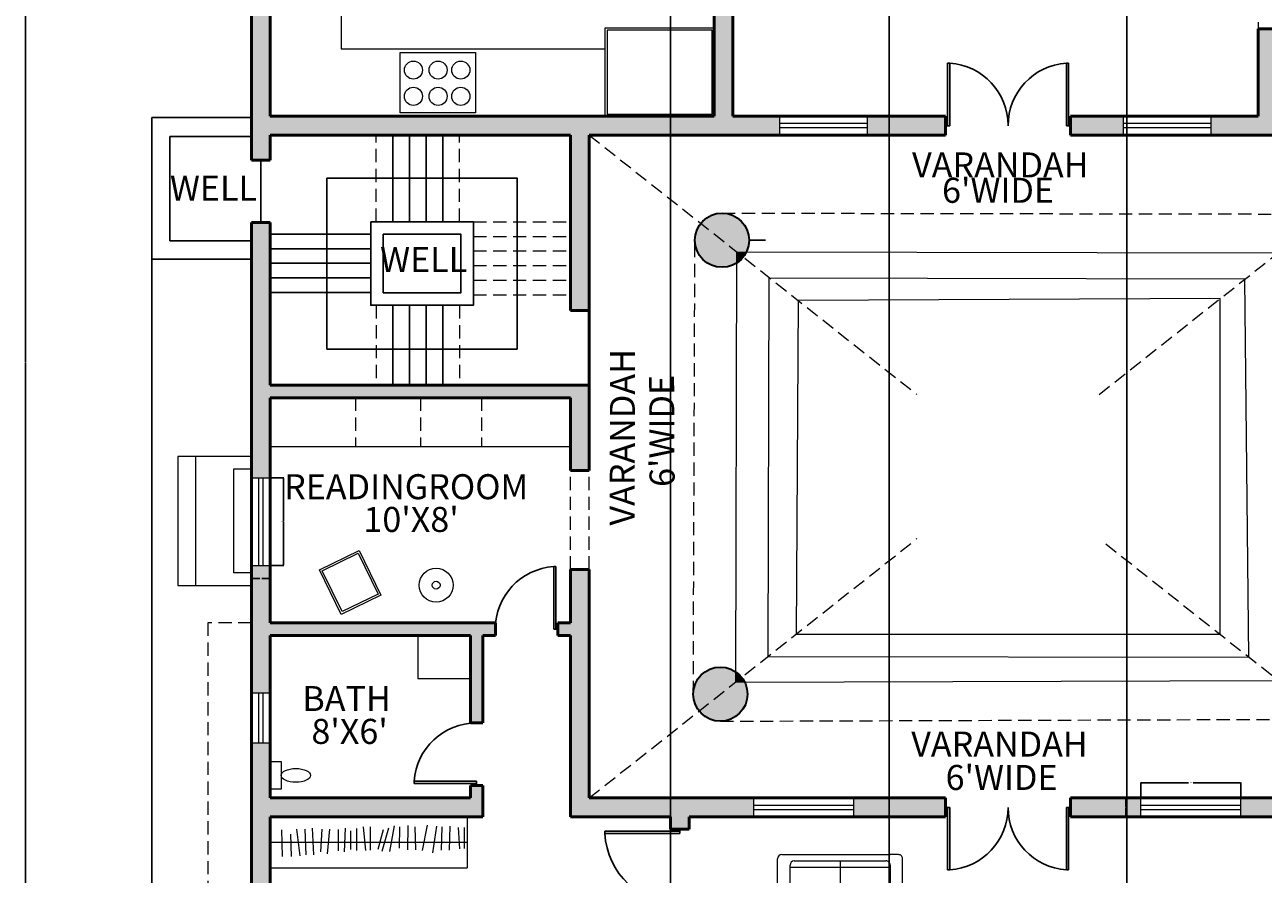
# Model space of a CAD drawing. Units: inches. Extents: x 2743 to 3669, y 1014 to 2282.
# Tile 2 of 5: x 2743 to 3337, y 1403 to 1810. Entities that reach past the tile are written whole.
import ezdxf

# ---------------------------------------------------------------- set-up
doc = ezdxf.new("R2010")
doc.units = ezdxf.units.IN
doc.linetypes.add('DASHED2', pattern=[9.525, 6.35, -3.175])
for name, color, linetype, lineweight in [('A-ANNO-DIMS', 2, 'Continuous', 18), ('A-ANNO-TEXT', 4, 'Continuous', 18), ('A-AREA-IDEN', 4, 'Continuous', 18), ('A-COLS', 7, 'Continuous', 35), ('A-DOOR', 211, 'Continuous', 25), ('A-EQPM', 51, 'Continuous', 18), ('A-FLOR-CASE', 51, 'Continuous', 18), ('A-FLOR-CASE-OVHD', 8, 'DASHED2', 13), ('A-FLOR-STRS', 7, 'Continuous', 25), ('A-FLOR-STRS-OVHD', 8, 'DASHED2', 18), ('A-FURN', 111, 'Continuous', 18), ('A-GLAZ', 40, 'Continuous', 20), ('A-ROOF', 7, 'Continuous', 20), ('A-ROOF-OVHD', 8, 'DASHED2', 18), ('A-WALL', 7, 'Continuous', 50), ('A-WALL-OVHD', 8, 'DASHED2', 18), ('P-EQPM', 4, 'Continuous', 25)]:
    doc.layers.add(name, color=color, linetype=linetype, lineweight=lineweight)
for name, color, linetype, lineweight, true_color in [('A-COLS-PATT', 47, 'Continuous', 13, 0x726c55), ('A-FLOR-FIXT', 11, 'Continuous', 18, 0xee778f), ('A-WALL-PATT', 47, 'Continuous', 13, 0x726c55)]:
    doc.layers.add(name, color=color, linetype=linetype, lineweight=lineweight, true_color=true_color)
doc.styles.get("Standard").update_dxf_attribs({"font": 'arial.ttf'})
doc.dimstyles.get("Standard").update_dxf_attribs({"dimtxt": 0.18, "dimasz": 0.18, "dimexe": 0.18, "dimexo": 0.0625, "dimgap": 0.09, "dimtad": 0, "dimtih": 1, "dimtoh": 1, "dimdec": 4, "dimzin": 0, "dimdsep": 46, "dimtxsty": 'Standard', "dimcen": 0.09, "dimadec": 0, "dimazin": 0, "dimtfac": 1, "dimtdec": 4, "dimtofl": 0, "dimtmove": 0, "dimatfit": 3, "dimfxl": 1, "dimtolj": 1, "dimtzin": 0, "dimarcsym": 0})

# ---------------------------------------------------------------- blocks, each defined once
blk = doc.blocks.new('DOOR-PAIR-60IN')
for p, q in [((0, 30), (1, 30)), ((1, 30), (1, 0)), ((2, 30), (1, 30)), ((2, 0), (2, 30)), ((58, 0), (58, 30)), ((58, 30), (59, 30)), ((60, 30), (59, 30)), ((59, 30), (59, 0)), ((1, 0), (2, 0)), ((59, 0), (58, 0))]:
    blk.add_line(p, q)
for centre, start, end in [((0, 29.93), 273.82241, 0.12746), ((60, 29.93), 179.99998, 266.1773)]:
    blk.add_arc(centre, 30, start, end)
blk = doc.blocks.new('DOOR-SINGLE-30IN')
for p, q in [((1, 0), (1, 30)), ((1, 30), (2, 30)), ((2, 30), (2, 0)), ((0, 0), (1, 0)), ((2, 0), (1, 0))]:
    blk.add_line(p, q)
blk.add_arc((0, 0.07), 30, 359.87254, 86.17759)
blk = doc.blocks.new('DOOR-SINGLE-36IN')
for p, q in [((1, 0), (1, 36)), ((1, 36), (2, 36)), ((2, 36), (2, 0)), ((0, 0), (1, 0)), ((2, 0), (1, 0))]:
    blk.add_line(p, q)
blk.add_arc((0, 0.06), 36, 359.91152, 86.81533)
blk = doc.blocks.new('WINDOW-24IN')
for p, q in [((0, 9), (0, 0)), ((24, 9), (24, 0)), ((0, 5.5), (24, 5.5)), ((0, 3.5), (24, 3.5))]:
    blk.add_line(p, q)
blk = doc.blocks.new('WINDOW-42IN')
for p, q in [((0, 42), (9, 42)), ((3.5, 0), (3.5, 42)), ((5.5, 0), (5.5, 42)), ((0, 0), (9, 0))]:
    blk.add_line(p, q)
blk = doc.blocks.new('WINDOW-48IN')
for p, q in [((0, 0), (0, 9)), ((48, 0), (48, 9)), ((0, 5.5), (48, 5.5)), ((0, 3.5), (48, 3.5))]:
    blk.add_line(p, q)
blk = doc.blocks.new('SOFA-TWO-SEAT')
for p, q in [((5, 60), (31, 60)), ((2, 54), (28, 54)), ((3, 54), (3, 58)), ((27, 54), (27, 6)), ((33, 58), (33, 6)), ((0, 32), (0, 52)), ((30, 52), (30, 8)), ((30, 30), (2, 30)), ((2, 30), (2, 30)), ((0, 28), (0, 8)), ((28, 6), (2, 6)), ((2, 6), (2, 6)), ((3, 6), (3, 2)), ((33, 2), (33, 6)), ((5, 0), (31, 0))]:
    blk.add_line(p, q)
for centre, start, end in [((5, 58), 90, 180), ((31, 58), 0, 90), ((2, 52), 90, 180), ((28, 52), 0, 90), ((2, 32), 180, 270), ((2, 28), 90, 180), ((2, 8), 180, 270), ((28, 8), 270, 0), ((5, 2), 180, 270), ((31, 2), 270, 0)]:
    blk.add_arc(centre, 2, start, end)
blk = doc.blocks.new('WC')
blk.add_lwpolyline([(0, 13.38), (5.3, 13.38), (5.3, 0), (0, 0)], close=True)
blk.add_ellipse((12.29, 6.69), major_axis=(7.08, 0), ratio=0.464281)
blk = doc.blocks.new('POST-COURTYARD')
blk.add_circle((13, 13), 13)
blk = doc.blocks.new('*D36')
at = {"layer": 'A-ANNO-DIMS', "color": 0, "lineweight": -2, "transparency": 16777216}
for p, q in [((2860.86, 1592.68), (2867.28, 1592.68)), ((2867.1, 1592.5), (2867.1, 1571.86)), ((2867.1, 1550.86), (2867.1, 1571.5)), ((2860.86, 1550.68), (2867.28, 1550.68))]:
    blk.add_line(p, q, dxfattribs=at)
at = {"layer": 'A-ANNO-DIMS', "color": 0, "transparency": 16777216}
for points in [[(2867.07, 1592.5), (2867.13, 1592.5), (2867.1, 1592.68)], [(2867.07, 1550.86), (2867.13, 1550.86), (2867.1, 1550.68)]]:
    blk.add_solid(points, dxfattribs=at)
at = {"layer": 'Defpoints', "color": 0, "transparency": 16777216}
for p in [(2860.8, 1592.68), (2867.1, 1592.68), (2860.8, 1550.68)]:
    blk.add_point(p, dxfattribs=at)
at = {"layer": 'A-ANNO-DIMS', "color": 0, "transparency": 16777216, "insert": (2867.1, 1571.68), "char_height": 0.18, "attachment_point": 5}
blk.add_mtext('\\A1;WINDOW 42 TYP.', dxfattribs=at)
blk = doc.blocks.new('*D37')
at = {"layer": 'A-ANNO-DIMS', "color": 0, "lineweight": -2, "transparency": 16777216}
for p, q in [((2851.8, 1550.62), (2851.8, 1544.2)), ((2860.8, 1550.62), (2860.8, 1544.2)), ((2851.98, 1544.38), (2855.84, 1544.38)), ((2860.62, 1544.38), (2856.75, 1544.38))]:
    blk.add_line(p, q, dxfattribs=at)
at = {"layer": 'A-ANNO-DIMS', "color": 0, "transparency": 16777216}
for points in [[(2851.98, 1544.41), (2851.98, 1544.35), (2851.8, 1544.38)], [(2860.62, 1544.41), (2860.62, 1544.35), (2860.8, 1544.38)]]:
    blk.add_solid(points, dxfattribs=at)
at = {"layer": 'Defpoints', "color": 0, "transparency": 16777216}
for p in [(2851.8, 1550.68), (2860.8, 1550.68), (2860.8, 1544.38)]:
    blk.add_point(p, dxfattribs=at)
at = {"layer": 'A-ANNO-DIMS', "color": 0, "transparency": 16777216, "insert": (2856.3, 1544.38), "char_height": 0.18, "attachment_point": 5}
blk.add_mtext('\\A1;9 TYP.', dxfattribs=at)
blk = doc.blocks.new('*D50')
at = {"layer": 'A-ANNO-DIMS', "color": 0, "lineweight": -2, "transparency": 16777216}
for p, q in [((3278.44, 1439.16), (3278.44, 1446.47)), ((3278.62, 1446.29), (3301.32, 1446.29)), ((3326.26, 1446.29), (3303.56, 1446.29)), ((3326.44, 1439.16), (3326.44, 1446.47))]:
    blk.add_line(p, q, dxfattribs=at)
at = {"layer": 'A-ANNO-DIMS', "color": 0, "transparency": 16777216}
for points in [[(3278.62, 1446.32), (3278.62, 1446.26), (3278.44, 1446.29)], [(3326.26, 1446.32), (3326.26, 1446.26), (3326.44, 1446.29)]]:
    blk.add_solid(points, dxfattribs=at)
at = {"layer": 'Defpoints', "color": 0, "transparency": 16777216}
for p in [(3326.44, 1446.29), (3278.44, 1439.09), (3326.44, 1439.09)]:
    blk.add_point(p, dxfattribs=at)
at = {"layer": 'A-ANNO-DIMS', "color": 0, "transparency": 16777216, "insert": (3302.44, 1446.29), "char_height": 0.18, "attachment_point": 5}
blk.add_mtext('\\A1;WINDOW 48 TYP.', dxfattribs=at)
blk = doc.blocks.new('*D51')
at = {"layer": 'A-ANNO-DIMS', "color": 0, "lineweight": -2, "transparency": 16777216}
for p, q in [((3278.38, 1439.09), (3271.06, 1439.09)), ((3271.24, 1438.91), (3271.24, 1434.78)), ((3271.24, 1430.27), (3271.24, 1434.41)), ((3278.38, 1430.09), (3271.06, 1430.09))]:
    blk.add_line(p, q, dxfattribs=at)
at = {"layer": 'A-ANNO-DIMS', "color": 0, "transparency": 16777216}
for points in [[(3271.21, 1438.91), (3271.27, 1438.91), (3271.24, 1439.09)], [(3271.21, 1430.27), (3271.27, 1430.27), (3271.24, 1430.09)]]:
    blk.add_solid(points, dxfattribs=at)
at = {"layer": 'Defpoints', "color": 0, "transparency": 16777216}
for p in [(3271.24, 1439.09), (3278.44, 1439.09), (3278.44, 1430.09)]:
    blk.add_point(p, dxfattribs=at)
at = {"layer": 'A-ANNO-DIMS', "color": 0, "transparency": 16777216, "insert": (3271.24, 1434.59), "char_height": 0.18, "attachment_point": 5}
blk.add_mtext('\\A1;9 TYP.', dxfattribs=at)
blk = doc.blocks.new('*D62')
at = {"layer": 'A-ANNO-DIMS', "color": 0, "lineweight": -2, "transparency": 16777216}
for p, q in [((3608.38, 1899.55), (3608.38, 1014.41)), ((2803.91, 1765.52), (2803.91, 1014.41)), ((2804.09, 1014.59), (3205.75, 1014.59)), ((3608.2, 1014.59), (3206.54, 1014.59))]:
    blk.add_line(p, q, dxfattribs=at)
at = {"layer": 'A-ANNO-DIMS', "color": 0, "transparency": 16777216}
for points in [[(2804.09, 1014.62), (2804.09, 1014.56), (2803.91, 1014.59)], [(3608.2, 1014.62), (3608.2, 1014.56), (3608.38, 1014.59)]]:
    blk.add_solid(points, dxfattribs=at)
at = {"layer": 'Defpoints', "color": 0, "transparency": 16777216}
for p in [(3608.38, 1899.61), (2803.91, 1765.58), (3608.38, 1014.59)]:
    blk.add_point(p, dxfattribs=at)
at = {"layer": 'A-ANNO-DIMS', "color": 0, "transparency": 16777216, "insert": (3206.15, 1014.59), "char_height": 0.18, "attachment_point": 5}
blk.add_mtext('\\A1;804.5', dxfattribs=at)
blk = doc.blocks.new('*D63')
at = {"layer": 'A-ANNO-DIMS', "color": 0, "lineweight": -2, "transparency": 16777216}
for p, q in [((3001.57, 2220.87), (2743.18, 2220.87)), ((2743.36, 2220.69), (2743.36, 1648.19)), ((2743.36, 1075.32), (2743.36, 1647.82)), ((3214.73, 1075.14), (2743.18, 1075.14))]:
    blk.add_line(p, q, dxfattribs=at)
at = {"layer": 'A-ANNO-DIMS', "color": 0, "transparency": 16777216}
for points in [[(2743.33, 2220.69), (2743.39, 2220.69), (2743.36, 2220.87)], [(2743.33, 1075.32), (2743.39, 1075.32), (2743.36, 1075.14)]]:
    blk.add_solid(points, dxfattribs=at)
at = {"layer": 'Defpoints', "color": 0, "transparency": 16777216}
for p in [(2743.36, 2220.87), (3001.63, 2220.87), (3214.8, 1075.14)]:
    blk.add_point(p, dxfattribs=at)
at = {"layer": 'A-ANNO-DIMS', "color": 0, "transparency": 16777216, "insert": (2743.36, 1648.01), "char_height": 0.18, "attachment_point": 5}
blk.add_mtext('\\A1;1145.7', dxfattribs=at)
blk = doc.blocks.new('*D76')
at = {"layer": 'A-ANNO-DIMS', "color": 0, "lineweight": -2, "transparency": 16777216}
for p, q in [((3052.84, 1130.9), (3052.84, 2281.6)), ((3053.02, 2281.42), (3104.86, 2281.42)), ((3157.62, 2281.42), (3105.77, 2281.42)), ((3157.8, 1130.9), (3157.8, 2281.6))]:
    blk.add_line(p, q, dxfattribs=at)
at = {"layer": 'A-ANNO-DIMS', "color": 0, "transparency": 16777216}
for points in [[(3053.02, 2281.45), (3053.02, 2281.39), (3052.84, 2281.42)], [(3157.62, 2281.45), (3157.62, 2281.39), (3157.8, 2281.42)]]:
    blk.add_solid(points, dxfattribs=at)
at = {"layer": 'Defpoints', "color": 0, "transparency": 16777216}
for p in [(3157.8, 2281.42), (3052.84, 1130.83), (3157.8, 1130.83)]:
    blk.add_point(p, dxfattribs=at)
at = {"layer": 'A-ANNO-DIMS', "color": 0, "transparency": 16777216, "insert": (3105.32, 2281.42), "char_height": 0.18, "attachment_point": 5}
blk.add_mtext('\\A1;104.95', dxfattribs=at)
blk = doc.blocks.new('*D77')
at = {"layer": 'A-ANNO-DIMS', "color": 0, "lineweight": -2, "transparency": 16777216}
for p, q in [((3157.8, 1130.9), (3157.8, 2281.6)), ((3157.98, 2281.42), (3214.52, 2281.42)), ((3271.62, 2281.42), (3215.08, 2281.42)), ((3271.8, 1130.9), (3271.8, 2281.6))]:
    blk.add_line(p, q, dxfattribs=at)
at = {"layer": 'A-ANNO-DIMS', "color": 0, "transparency": 16777216}
for points in [[(3157.98, 2281.45), (3157.98, 2281.39), (3157.8, 2281.42)], [(3271.62, 2281.45), (3271.62, 2281.39), (3271.8, 2281.42)]]:
    blk.add_solid(points, dxfattribs=at)
at = {"layer": 'Defpoints', "color": 0, "transparency": 16777216}
for p in [(3271.8, 2281.42), (3157.8, 1130.83), (3271.8, 1130.83)]:
    blk.add_point(p, dxfattribs=at)
at = {"layer": 'A-ANNO-DIMS', "color": 0, "transparency": 16777216, "insert": (3214.8, 2281.42), "char_height": 0.18, "attachment_point": 5}
blk.add_mtext('\\A1;114', dxfattribs=at)
blk = doc.blocks.new('*D78')
at = {"layer": 'A-ANNO-DIMS', "color": 0, "lineweight": -2, "transparency": 16777216}
for p, q in [((3271.8, 1130.9), (3271.8, 2281.6)), ((3271.98, 2281.42), (3323.82, 2281.42)), ((3376.57, 2281.42), (3324.73, 2281.42)), ((3376.75, 1130.9), (3376.75, 2281.6))]:
    blk.add_line(p, q, dxfattribs=at)
at = {"layer": 'A-ANNO-DIMS', "color": 0, "transparency": 16777216}
for points in [[(3271.98, 2281.45), (3271.98, 2281.39), (3271.8, 2281.42)], [(3376.57, 2281.45), (3376.57, 2281.39), (3376.75, 2281.42)]]:
    blk.add_solid(points, dxfattribs=at)
at = {"layer": 'Defpoints', "color": 0, "transparency": 16777216}
for p in [(3376.75, 2281.42), (3271.8, 1130.83), (3376.75, 1130.83)]:
    blk.add_point(p, dxfattribs=at)
at = {"layer": 'A-ANNO-DIMS', "color": 0, "transparency": 16777216, "insert": (3324.27, 2281.42), "char_height": 0.18, "attachment_point": 5}
blk.add_mtext('\\A1;104.95', dxfattribs=at)
blk = doc.blocks.new('*D80')
at = {"layer": 'A-ANNO-DIMS', "color": 0, "lineweight": -2, "transparency": 16777216}
for p, q in [((3077.46, 1706.66), (3077.64, 1706.66)), ((3077.55, 1706.57), (3077.55, 1706.75)), ((3098.35, 1706.66), (3090.73, 1706.66))]:
    blk.add_line(p, q, dxfattribs=at)
at = {"layer": 'A-ANNO-DIMS', "color": 0, "transparency": 16777216}
blk.add_solid([(3090.73, 1706.69), (3090.73, 1706.63), (3090.55, 1706.66)], dxfattribs=at)
at = {"layer": 'Defpoints', "color": 0, "transparency": 16777216}
for p in [(3064.55, 1706.66), (3090.55, 1706.66)]:
    blk.add_point(p, dxfattribs=at)
at = {"layer": 'A-ANNO-DIMS', "color": 0, "transparency": 16777216, "insert": (3098.86, 1706.66), "char_height": 0.18, "attachment_point": 5}
blk.add_mtext('\\A1;4X ∅26', dxfattribs=at)

msp = doc.modelspace()

# ---------------------------------------------------------------- hatches: boundary and pattern name
at = {"layer": 'A-COLS-PATT'}
h = msp.add_hatch(color=256, dxfattribs=at)
h.dxf.hatch_style = 1
h.paths.add_polyline_path([(3084.706, 1701.002), (3089.245, 1700.991, 0.1133638), (3090.548, 1706.664, 0.7110205), (3067.352, 1714.729)])
h = msp.add_hatch(color=256, dxfattribs=at)
h.dxf.hatch_style = 1
h.paths.add_polyline_path([(3084.471, 1695.66), (3084.484, 1701.177), (3067.352, 1714.729, 0.1688931), (3064.548, 1706.664, 0.5900785)])
h = msp.add_hatch(color=256, dxfattribs=at)
h.dxf.hatch_style = 1
h.paths.add_polyline_path([(3084.706, 1701.002), (3084.483, 1701.002), (3084.471, 1695.66, 0.0851969), (3087.744, 1698.598)])
h = msp.add_hatch(color=256, dxfattribs=at)
h.dxf.hatch_style = 1
h.paths.add_polyline_path([(3089.245, 1700.991), (3084.706, 1701.002), (3087.744, 1698.598, 0.054486)])
h = msp.add_hatch(color=256, dxfattribs=at)
h.dxf.hatch_style = 1
h.paths.add_polyline_path([(3084.008, 1494.635), (3084.02, 1499.684, 0.6005781), (3063.759, 1488.9, 0.1688931), (3066.563, 1480.835)])
h = msp.add_hatch(color=256, dxfattribs=at)
h.dxf.hatch_style = 1
h.paths.add_polyline_path([(3084.02, 1499.684), (3084.008, 1494.635), (3086.955, 1496.966, 0.0773936)])
h = msp.add_hatch(color=256, dxfattribs=at)
h.dxf.hatch_style = 1
h.paths.add_polyline_path([(3066.563, 1480.835, 0.7110205), (3089.759, 1488.9, 0.1150215), (3088.419, 1494.649), (3084.008, 1494.635)])
h = msp.add_hatch(color=256, dxfattribs=at)
h.dxf.hatch_style = 1
h.paths.add_polyline_path([(3086.955, 1496.966), (3084.008, 1494.635), (3088.419, 1494.649, 0.052845)])
at = {"layer": 'A-WALL-PATT'}
h = msp.add_hatch(color=256, dxfattribs=at)
h.dxf.hatch_style = 1
h.paths.add_polyline_path([(3082.796, 1838.094), (3073.796, 1838.094), (3073.796, 1766.094), (3021.39, 1766.094), (2860.796, 1766.094), (2860.796, 1827.347), (2851.796, 1827.347), (2851.796, 1745.094), (2860.796, 1745.094), (2860.796, 1757.094), (3004.796, 1757.094), (3004.796, 1672.878), (3013.796, 1672.878), (3013.796, 1757.094), (3105.339, 1757.094), (3105.339, 1766.094), (3082.796, 1766.094)])
h = msp.add_hatch(color=256, dxfattribs=at)
h.dxf.hatch_style = 1
h.paths.add_polyline_path([(3312.269, 1766.094), (3312.269, 1757.094), (3366.681, 1757.094), (3366.681, 1766.094), (3343.796, 1766.094), (3343.796, 1808.094), (3334.796, 1808.094), (3334.796, 1766.094)])
h = msp.add_hatch(color=256, dxfattribs=at)
h.dxf.hatch_style = 1
h.paths.add_polyline_path([(3184.796, 1757.094), (3184.796, 1766.094), (3147.339, 1766.094), (3147.339, 1757.094)])
h = msp.add_hatch(color=256, dxfattribs=at)
h.dxf.hatch_style = 1
h.paths.add_polyline_path([(3270.189, 1757.094), (3270.189, 1766.094), (3244.796, 1766.094), (3244.796, 1757.094)])
h = msp.add_hatch(color=256, dxfattribs=at)
h.dxf.hatch_style = 1
h.paths.add_polyline_path([(2860.796, 1715.094), (2851.796, 1715.094), (2851.796, 1592.679), (2860.796, 1592.679), (2860.796, 1631.094), (3004.796, 1631.094), (3004.796, 1596.185), (3013.796, 1596.185), (3013.796, 1637.094), (2860.796, 1637.094)])
h = msp.add_hatch(color=256, dxfattribs=at)
h.dxf.hatch_style = 1
h.paths.add_polyline_path([(3568.796, 1514.094), (3568.796, 1491.964), (3577.796, 1491.964), (3577.796, 1574.145), (3568.796, 1574.145), (3568.796, 1523.094), (3507.198, 1523.094), (3424.796, 1523.094), (3424.796, 1529.094), (3415.796, 1529.094), (3415.796, 1439.094), (3326.438, 1439.094), (3326.438, 1430.094), (3367.796, 1430.094), (3367.796, 1424.094), (3376.796, 1424.094), (3376.796, 1430.094), (3430.796, 1430.094), (3430.796, 1439.094), (3424.796, 1439.094), (3424.796, 1514.094), (3472.796, 1514.094), (3472.796, 1439.094), (3460.796, 1439.094), (3460.796, 1430.094), (3514.579, 1430.094), (3514.579, 1439.094), (3478.796, 1439.094), (3478.796, 1514.094)])
h = msp.add_hatch(color=256, dxfattribs=at)
h.dxf.hatch_style = 1
h.paths.add_polyline_path([(2851.796, 1489.516), (2860.796, 1489.516), (2860.796, 1517.094), (2956.796, 1517.094), (2956.796, 1496.461), (2956.796, 1475.094), (2962.796, 1475.094), (2962.796, 1517.094), (2968.796, 1517.094), (2968.796, 1523.094), (2860.796, 1523.094), (2860.796, 1550.679), (2851.796, 1550.679)])
h = msp.add_hatch(color=256, dxfattribs=at)
h.dxf.hatch_style = 1
h.paths.add_polyline_path([(3052.796, 1430.094), (3052.796, 1424.094), (3061.796, 1424.094), (3061.796, 1430.094), (3092.842, 1430.094), (3092.842, 1439.094), (3013.796, 1439.094), (3013.796, 1548.663), (3004.796, 1548.663), (3004.796, 1523.094), (2998.796, 1523.094), (2998.796, 1517.094), (3004.796, 1517.094), (3004.796, 1430.094)])
h = msp.add_hatch(color=256, dxfattribs=at)
h.dxf.hatch_style = 1
h.paths.add_polyline_path([(2851.796, 1356.075), (2856.296, 1356.075), (2860.796, 1356.075), (2860.796, 1360.685), (2860.796, 1380.133), (2860.796, 1430.094), (2955.206, 1430.094), (2962.796, 1430.094), (2962.796, 1445.094), (2956.796, 1445.094), (2956.796, 1439.094), (2860.796, 1439.094), (2860.796, 1443.244), (2860.771, 1443.244), (2860.771, 1456.626), (2860.775, 1465.516), (2851.796, 1465.516)])
h = msp.add_hatch(color=256, dxfattribs=at)
h.dxf.hatch_style = 1
h.paths.add_polyline_path([(3140.842, 1439.094), (3140.842, 1430.094), (3184.796, 1430.094), (3184.796, 1439.094)])
h = msp.add_hatch(color=256, dxfattribs=at)
h.dxf.hatch_style = 1
h.paths.add_polyline_path([(3244.796, 1439.094), (3244.796, 1430.094), (3278.438, 1430.094), (3278.438, 1439.094)])

# ---------------------------------------------------------------- linework, layer by layer
at = {"layer": 'A-EQPM'}
msp.add_lwpolyline([(2923.115, 1796.685), (2959.239, 1796.685), (2959.239, 1767.715), (2923.115, 1767.715)], close=True, dxfattribs=at)
for centre in [(2929.481, 1788.263), (2941.316, 1788.263), (2952.206, 1788.263), (2929.481, 1775.684), (2941.316, 1775.684), (2952.206, 1775.684)]:
    msp.add_circle(centre, 4.34, dxfattribs=at)
at = {"layer": 'A-FLOR-CASE'}
for p, q in [((2894.795, 1937.562), (2894.795, 1798.541)), ((2894.795, 1798.541), (3021.39, 1798.541)), ((3004.796, 1607.482), (2860.796, 1607.482)), ((2955.206, 1430.094), (2955.206, 1405.612)), ((2866.137, 1423.741), (2866.495, 1411.043)), ((2870.97, 1411.043), (2870.671, 1421.657)), ((2873.297, 1424.099), (2874.908, 1411.401)), ((2877.414, 1424.099), (2877.772, 1411.758)), ((2880.815, 1424.636), (2881.58, 1411.869)), ((2885.469, 1424.099), (2884.932, 1413.189)), ((2889.228, 1424.099), (2888.154, 1412.295)), ((2893.346, 1423.92), (2893.346, 1413.726)), ((2896.747, 1424.636), (2896.21, 1413.189)), ((2899.253, 1423.384), (2899.253, 1414.441)), ((2902.117, 1424.457), (2902.117, 1413.905)), ((2905.339, 1425.172), (2906.413, 1413.905)), ((2908.74, 1425.172), (2908.74, 1414.083)), ((2915.005, 1423.741), (2912.32, 1414.441)), ((2917.511, 1424.636), (2914.254, 1413.354)), ((2920.196, 1425.709), (2918.048, 1413.354)), ((2922.749, 1425.265), (2922.702, 1414.978)), ((2926.819, 1425.888), (2926.64, 1414.262)), ((2930.22, 1425.172), (2930.404, 1414.204)), ((2936.128, 1426.066), (2933.622, 1413.905)), ((2940.603, 1425.53), (2938.634, 1412.832)), ((2943.109, 1425.172), (2942.751, 1414.083)), ((2946.868, 1425.53), (2946.689, 1414.083)), ((2950.985, 1424.993), (2951.522, 1414.62)), ((2953.849, 1424.993), (2953.849, 1414.799)), ((2860.796, 1417.853), (2955.206, 1417.853))]:
    msp.add_line(p, q, dxfattribs=at)
for points in [[(3073.796, 1808.417), (3021.39, 1808.417), (3021.39, 1766.094), (3073.796, 1766.094)], [(3072.796, 1807.417), (3022.39, 1807.417), (3022.39, 1767.094), (3072.796, 1767.094)]]:
    msp.add_lwpolyline(points, close=True, dxfattribs=at)
msp.add_lwpolyline([(2955.206, 1430.094), (2860.796, 1430.094), (2860.796, 1405.612), (2955.206, 1405.612)], dxfattribs=at)
at = {"layer": 'A-FLOR-CASE-OVHD'}
for p, q in [((2901.733, 1631.094), (2901.733, 1607.482)), ((2932.796, 1631.094), (2932.796, 1607.482)), ((2962.169, 1631.094), (2962.169, 1607.482))]:
    msp.add_line(p, q, dxfattribs=at)
at = {"layer": 'A-FLOR-FIXT'}
msp.add_lwpolyline([(2956.796, 1517.094), (2931.603, 1517.094), (2931.603, 1496.461), (2956.796, 1496.461)], close=True, dxfattribs=at)
at = {"layer": 'A-FLOR-STRS'}
for p, q in [((2851.796, 1765.581), (2803.91, 1765.581)), ((2803.91, 1765.581), (2803.91, 1697.511)), ((2851.796, 1756.376), (2812.638, 1756.376)), ((2812.638, 1756.376), (2812.638, 1706.376)), ((2919.563, 1715.5), (2919.563, 1757.094)), ((2927.563, 1715.5), (2927.563, 1757.094)), ((2935.563, 1715.5), (2935.563, 1757.094)), ((2943.563, 1715.5), (2943.563, 1757.094)), ((2856.296, 1745.094), (2856.296, 1715.094)), ((2812.638, 1706.376), (2851.796, 1706.376)), ((2860.796, 1709.603), (2908.965, 1709.603)), ((2860.796, 1702.603), (2908.965, 1702.603)), ((2803.91, 1697.511), (2851.796, 1697.511)), ((2860.796, 1695.603), (2908.965, 1695.603)), ((2860.796, 1688.603), (2908.965, 1688.603)), ((2860.796, 1681.603), (2908.965, 1681.603)), ((2919.563, 1675.424), (2919.563, 1637.094)), ((2927.563, 1675.424), (2927.563, 1637.094)), ((2935.563, 1675.424), (2935.563, 1637.094)), ((2943.563, 1675.424), (2943.563, 1637.094))]:
    msp.add_line(p, q, dxfattribs=at)
msp.add_lwpolyline([(2887.965, 1736.5), (2979.239, 1736.5), (2979.239, 1654.424), (2887.965, 1654.424)], close=True, dxfattribs=at)
at = {"layer": 'A-FLOR-STRS-OVHD'}
for p, q in [((2911.563, 1715.5), (2911.563, 1757.094)), ((2951.563, 1715.5), (2951.563, 1757.094)), ((2958.239, 1715.5), (3004.796, 1715.5)), ((2958.239, 1708.5), (3004.796, 1708.5)), ((2958.239, 1701.5), (3004.796, 1701.5)), ((2958.239, 1694.5), (3004.796, 1694.5)), ((2958.239, 1687.5), (3004.796, 1687.5)), ((2958.239, 1680.5), (3004.796, 1680.5)), ((2911.563, 1675.424), (2911.563, 1637.094)), ((2951.563, 1675.424), (2951.563, 1637.094))]:
    msp.add_line(p, q, dxfattribs=at)
at = {"layer": 'A-FURN'}
for points in [[(2884.405, 1548.504), (2903.435, 1557.792), (2913.859, 1536.435), (2894.829, 1527.148)], [(2885.743, 1548.044), (2902.975, 1556.455), (2912.521, 1536.895), (2895.289, 1528.485)]]:
    msp.add_lwpolyline(points, close=True, dxfattribs=at)
for radius in [8.161, 1.875]:
    msp.add_circle((2940.365, 1541.169), radius, dxfattribs=at)
at = {"layer": 'A-GLAZ'}
for p, q in [((2843.363, 1547.135), (2843.363, 1596.97)), ((2843.363, 1596.97), (2851.796, 1596.97)), ((2851.796, 1547.135), (2843.363, 1547.135))]:
    msp.add_line(p, q, dxfattribs=at)
at = {"layer": 'A-ROOF'}
for p, q in [((3084.484, 1701.177), (3084.008, 1494.635)), ((3344.132, 1700.404), (3084.483, 1701.002)), ((3099.966, 1688.93), (3099.575, 1506.949)), ((3328.383, 1687.946), (3099.965, 1688.436)), ((3330.345, 1506.69), (3328.383, 1687.946)), ((3114.148, 1677.712), (3113.076, 1517.629)), ((3316.611, 1678.634), (3114.148, 1677.712)), ((3316.549, 1517.603), (3316.611, 1678.634)), ((2851.796, 1602.97), (2816.503, 1602.97)), ((2816.503, 1602.97), (2816.503, 1540.97)), ((2825.007, 1540.97), (2825.007, 1602.97)), ((2851.796, 1596.97), (2851.796, 1602.97)), ((2816.503, 1540.97), (2851.796, 1540.97)), ((3113.076, 1517.629), (3316.549, 1517.603)), ((3099.575, 1506.949), (3330.345, 1506.69)), ((3084.008, 1494.635), (3344.492, 1495.499))]:
    msp.add_line(p, q, dxfattribs=at)
at = {"layer": 'A-ROOF-OVHD'}
for p, q in [((3013.796, 1757.094), (3171.076, 1632.679)), ((3258.517, 1632.679), (3415.796, 1757.094)), ((3077.548, 1719.664), (3351.487, 1719.206)), ((3063.759, 1488.9), (3064.548, 1706.664)), ((3013.796, 1439.094), (3171.076, 1563.509)), ((3261.659, 1561.024), (3415.796, 1439.094)), ((2851.796, 1523.146), (2830.796, 1523.146)), ((2830.796, 1523.146), (2830.796, 1360.075)), ((3076.759, 1475.9), (3351.466, 1476.837))]:
    msp.add_line(p, q, dxfattribs=at)
at = {"layer": 'A-WALL'}
for p, q in [((2860.796, 1766.094), (2860.796, 1958.094)), ((3073.796, 1766.094), (3073.796, 1838.094)), ((3082.796, 1766.094), (3082.796, 1838.094)), ((3334.796, 1766.094), (3334.796, 1808.094)), ((3334.796, 1808.094), (3343.796, 1808.094)), ((2860.796, 1766.094), (3073.796, 1766.094)), ((3082.796, 1766.094), (3184.796, 1766.094)), ((3184.796, 1766.094), (3184.796, 1757.094)), ((3244.796, 1766.094), (3244.796, 1757.094)), ((3244.796, 1766.094), (3334.796, 1766.094)), ((2860.796, 1757.094), (3004.796, 1757.094)), ((2860.796, 1757.094), (2860.796, 1745.094)), ((2860.796, 1745.094), (2860.796, 1757.094)), ((3004.796, 1672.878), (3004.796, 1757.094)), ((3013.796, 1757.094), (3184.796, 1757.094)), ((3013.796, 1596.185), (3013.796, 1757.094)), ((3244.796, 1757.094), (3415.796, 1757.094)), ((2860.796, 1745.094), (2851.796, 1745.094)), ((2860.796, 1715.094), (2851.796, 1715.094)), ((2860.796, 1637.094), (2860.796, 1715.094)), ((3004.796, 1672.878), (3013.796, 1672.878)), ((2860.796, 1637.094), (3013.796, 1637.094)), ((2860.796, 1631.094), (3004.796, 1631.094)), ((2860.796, 1523.094), (2860.796, 1631.094)), ((3004.796, 1596.185), (3004.796, 1631.094)), ((3004.796, 1596.185), (3013.796, 1596.185)), ((3004.796, 1523.094), (3004.796, 1548.663)), ((3004.796, 1548.663), (3013.796, 1548.663)), ((3013.796, 1439.094), (3013.796, 1548.663)), ((2860.796, 1523.094), (2968.796, 1523.094)), ((2968.796, 1517.094), (2968.796, 1523.094)), ((2998.796, 1517.094), (2998.796, 1523.094)), ((2998.796, 1523.094), (3004.796, 1523.094)), ((2860.796, 1439.094), (2860.796, 1517.094)), ((2860.796, 1517.094), (2956.796, 1517.094)), ((2956.796, 1475.094), (2956.796, 1517.094)), ((2962.796, 1517.094), (2968.796, 1517.094)), ((2962.796, 1475.094), (2962.796, 1517.094)), ((3004.796, 1517.094), (2998.796, 1517.094)), ((2998.796, 1517.094), (3004.796, 1517.094)), ((3004.796, 1430.094), (3004.796, 1517.094)), ((2956.796, 1475.094), (2962.796, 1475.094)), ((2956.796, 1439.094), (2956.796, 1445.094)), ((2956.796, 1445.094), (2962.796, 1445.094)), ((2962.796, 1430.094), (2962.796, 1445.094)), ((2956.796, 1439.094), (2860.796, 1439.094)), ((3184.796, 1439.094), (3013.796, 1439.094)), ((3184.796, 1439.094), (3184.796, 1430.094)), ((3415.796, 1439.094), (3244.796, 1439.094)), ((3244.796, 1439.094), (3244.796, 1430.094)), ((2860.796, 1238.094), (2860.796, 1430.094)), ((2962.796, 1430.094), (2860.796, 1430.094)), ((3052.796, 1430.094), (3004.796, 1430.094)), ((3052.796, 1424.094), (3052.796, 1430.094)), ((3061.796, 1424.094), (3061.796, 1430.094)), ((3184.796, 1430.094), (3061.796, 1430.094)), ((3367.796, 1430.094), (3244.796, 1430.094)), ((3052.796, 1424.094), (3061.796, 1424.094))]:
    msp.add_line(p, q, dxfattribs=at)
for points in [[(2851.796, 1745.094), (2851.796, 1991.094)], [(2851.796, 1356.075), (2851.796, 1715.094)]]:
    msp.add_lwpolyline(points, dxfattribs=at)
at = {"layer": 'A-WALL-OVHD'}
for p, q in [((3334.796, 1916.094), (3334.796, 1808.094)), ((3004.796, 1548.663), (3004.796, 1596.185)), ((3013.796, 1548.663), (3013.796, 1596.185))]:
    msp.add_line(p, q, dxfattribs=at)
at = {"layer": 'P-EQPM'}
for points in [[(2908.965, 1715.5), (2958.239, 1715.5), (2958.239, 1675.424), (2908.965, 1675.424)], [(2914.965, 1709.5), (2952.239, 1709.5), (2952.239, 1681.424), (2914.965, 1681.424)]]:
    msp.add_lwpolyline(points, close=True, dxfattribs=at)

# ---------------------------------------------------------------- block references
at = {"layer": 'A-COLS'}
for p in [(3064.548, 1693.664), (3063.759, 1475.901)]:
    msp.add_blockref('POST-COURTYARD', p, dxfattribs=at)
at = {"layer": 'A-DOOR'}
for name, p, rotation in [('DOOR-PAIR-60IN', (3244.796, 1791.594), 180.0036176401362), ('DOOR-SINGLE-30IN', (2959.797, 1445.094), 89.99999999999827), ('DOOR-PAIR-60IN', (3184.795, 1404.593), 359.9963984722729)]:
    msp.add_blockref(name, p, dxfattribs=dict(at, rotation=rotation))
at = {"layer": 'A-DOOR', "extrusion": (0, 0, -1), "zscale": -1}
msp.add_blockref('DOOR-SINGLE-30IN', (-2998.797, 1520.094), dxfattribs=at)
at = {"layer": 'A-DOOR', "extrusion": (0, 0, -1), "zscale": -1, "rotation": 270.0000000000017}
msp.add_blockref('DOOR-SINGLE-36IN', (-3057.297, 1424.095), dxfattribs=at)
at = {"layer": 'A-FLOR-FIXT'}
msp.add_blockref('WC', (2860.771, 1443.244), dxfattribs=at)
at = {"layer": 'A-FURN', "rotation": 90.00000000000146}
msp.add_blockref('SOFA-TWO-SEAT', (3164.19, 1378.923), dxfattribs=at)
at = {"layer": 'A-GLAZ'}
for name, p, rotation in [('WINDOW-42IN', (3147.339, 1757.094), 89.9999999999987), ('WINDOW-42IN', (3312.23, 1757.102), 90.02243882400342), ('WINDOW-24IN', (2860.797, 1465.516), 90.00000000000144)]:
    msp.add_blockref(name, p, dxfattribs=dict(at, rotation=rotation))
for name, p in [('WINDOW-42IN', (2851.796, 1550.679)), ('WINDOW-48IN', (3092.842, 1430.094)), ('WINDOW-48IN', (3278.438, 1430.094))]:
    msp.add_blockref(name, p, dxfattribs=at)

# ---------------------------------------------------------------- texts
at = {"layer": 'A-ANNO-TEXT'}
for p in [(2812.638, 1725.647), (2913.489, 1691.332)]:
    msp.add_attdef('WELL', p, '', height=12, dxfattribs=at)
at = {"layer": 'A-AREA-IDEN'}
for tag, p in [('VARANDAH', (3168.735, 1736.772)), ("6'WIDE", (3183.132, 1724.601)), ('READINGROOM', (2867.411, 1582.412)), ("10'X8'", (2905.478, 1566.707)), ('BATH', (2876.168, 1480.816)), ("8'X6'", (2880.527, 1465.024)), ('VARANDAH', (3168.341, 1458.936)), ("6'WIDE", (3184.83, 1442.933))]:
    msp.add_attdef(tag, p, '', height=12, dxfattribs=at)
for tag, p, rotation in [('VARANDAH', (3035.65, 1569.748), 89.904183), ("6'WIDE", (3054.803, 1588.346), 90.261085)]:
    msp.add_attdef(tag, p, '', height=12, rotation=rotation, dxfattribs=at)

# ---------------------------------------------------------------- dimensions: what is measured, and where the dimension line sits
at = {"layer": 'A-ANNO-DIMS'}
for base, p1, p2, override, picture, middle in [((3157.796, 2281.421), (3052.842, 1130.835), (3157.796, 1130.835), {"dimdec": 2, "dimlfac": 1, "dimrnd": 0, "dimzin": 0, "dimdsep": 46, "dimlunit": 2}, '*D76', (3105.319, 2281.421)), ((3271.796, 2281.421), (3157.796, 1130.835), (3271.796, 1130.835), {"dimdec": 0, "dimlfac": 1, "dimrnd": 0, "dimzin": 0, "dimdsep": 46, "dimlunit": 2}, '*D77', (3214.796, 2281.421)), ((3376.7513, 2281.4212), (3271.7965, 1130.8347), (3376.7513, 1130.8347), {"dimdec": 2, "dimlfac": 1, "dimrnd": 0, "dimzin": 0, "dimdsep": 46, "dimlunit": 2}, '*D78', (3324.2739, 2281.4212)), ((3608.383, 1014.589), (2803.91, 1765.581), (3608.383, 1899.608), {"dimdec": 1, "dimlfac": 1, "dimrnd": 0, "dimzin": 0, "dimdsep": 46, "dimlunit": 2}, '*D62', (3206.146, 1014.589))]:
    dim = msp.add_linear_dim(base=base, p1=p1, p2=p2, dimstyle='Standard', override=override, dxfattribs=at)
    dim.commit()
    dim.dimension.update_dxf_attribs({"geometry": picture, "text_midpoint": middle})
dim = msp.add_linear_dim(base=(2743.36, 2220.871), p1=(3214.796, 1075.139), p2=(3001.629, 2220.871), angle=90, dimstyle='Standard', override={"dimdec": 1, "dimlfac": 1, "dimrnd": 0, "dimzin": 0, "dimdsep": 46, "dimlunit": 2}, dxfattribs=at)
dim.commit()
dim.dimension.update_dxf_attribs({"geometry": '*D63', "text_midpoint": (2743.36, 1648.005)})
dim = msp.add_diameter_dim_2p(p1=(3064.548, 1706.663), p2=(3090.548, 1706.664), text='4X <>', dimstyle='Standard', override={"dimdec": 0, "dimlfac": 1, "dimrnd": 0, "dimzin": 0, "dimdsep": 46, "dimlunit": 2}, dxfattribs=at)
dim.commit()
dim.dimension.update_dxf_attribs({"geometry": '*D80', "text_midpoint": (3098.348, 1706.664), "dimtype": 163})
for base, p1, p2, text, picture, middle in [((2867.096, 1592.679), (2860.796, 1550.679), (2860.796, 1592.679), 'WINDOW <> TYP.', '*D36', (2867.096, 1571.679)), ((3271.238, 1439.094), (3278.438, 1430.094), (3278.438, 1439.094), '<> TYP.', '*D51', (3271.238, 1434.594))]:
    dim = msp.add_linear_dim(base=base, p1=p1, p2=p2, angle=90, text=text, dimstyle='Standard', override={"dimdec": 0, "dimlfac": 1, "dimrnd": 0, "dimzin": 0, "dimdsep": 46, "dimlunit": 2}, dxfattribs=at)
    dim.commit()
    dim.dimension.update_dxf_attribs({"geometry": picture, "text_midpoint": middle})
for base, p1, p2, text, picture, middle in [((2860.796, 1544.379), (2851.796, 1550.679), (2860.796, 1550.679), '<> TYP.', '*D37', (2856.296, 1544.379)), ((3326.438, 1446.294), (3278.438, 1439.094), (3326.438, 1439.094), 'WINDOW <> TYP.', '*D50', (3302.438, 1446.294))]:
    dim = msp.add_linear_dim(base=base, p1=p1, p2=p2, text=text, dimstyle='Standard', override={"dimdec": 0, "dimlfac": 1, "dimrnd": 0, "dimzin": 0, "dimdsep": 46, "dimlunit": 2}, dxfattribs=at)
    dim.commit()
    dim.dimension.update_dxf_attribs({"geometry": picture, "text_midpoint": middle})

doc.saveas('drawing.dxf')
